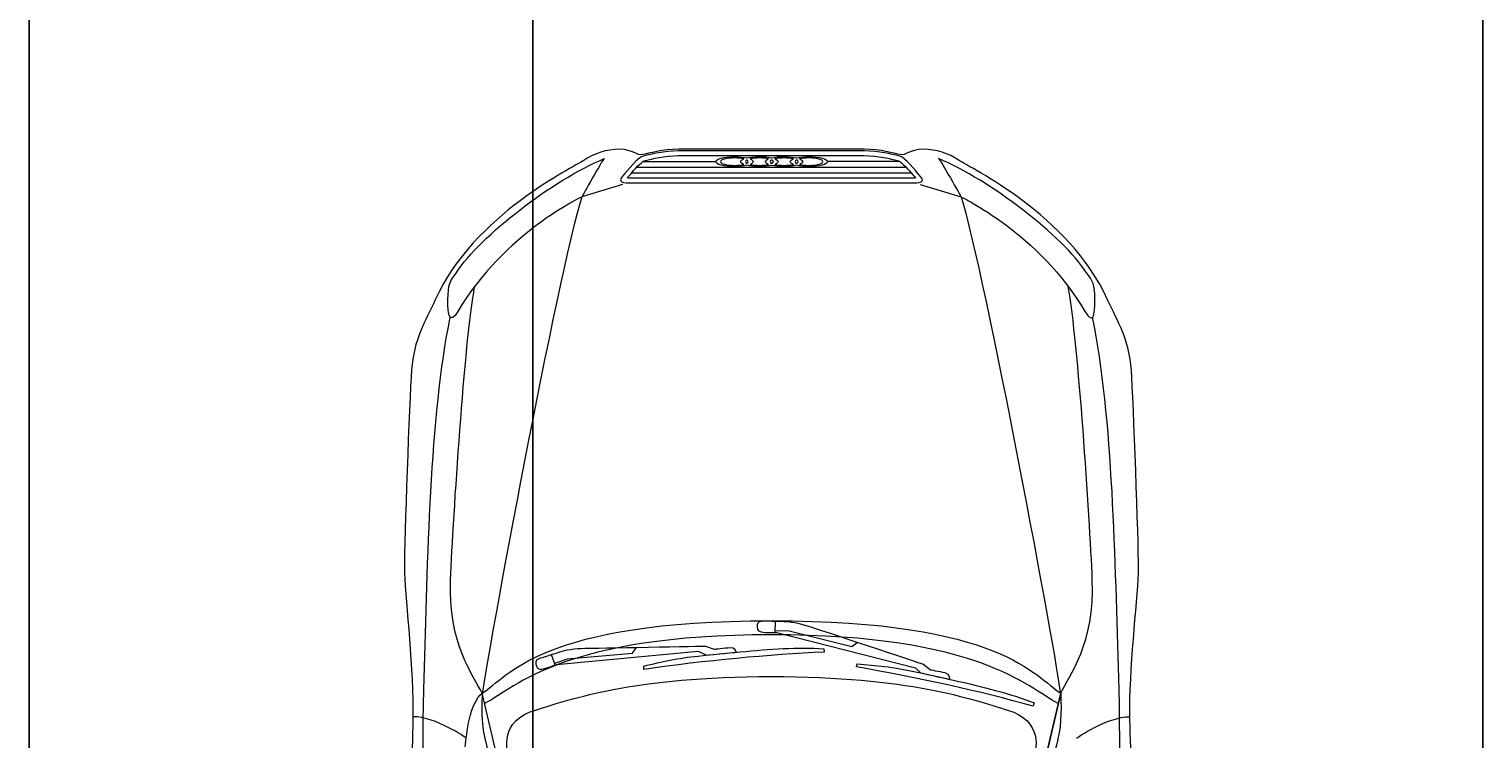
# Model space of a CAD drawing. Units: inches. Extents: x 1734 to 2405, y 1500 to 2491.
# Tile 5 of 14: x 1798 to 1875, y 1851 to 1888. Entities that reach past the tile are written whole.
import ezdxf

# ---------------------------------------------------------------- set-up
doc = ezdxf.new("R2010")
doc.units = ezdxf.units.IN
for name, color, linetype, lineweight in [('A-ANNO-DIMS', 2, 'Continuous', 18), ('AUDI', 8, 'Continuous', 18), ('C-PROP', 7, 'Continuous', 25)]:
    doc.layers.add(name, color=color, linetype=linetype, lineweight=lineweight)
doc.styles.get("Standard").update_dxf_attribs({"font": 'arial.ttf'})
doc.dimstyles.get("Standard").update_dxf_attribs({"dimtxt": 0.18, "dimasz": 0.18, "dimexe": 0.18, "dimexo": 0.0625, "dimgap": 0.09, "dimtad": 0, "dimtih": 1, "dimtoh": 1, "dimdec": 4, "dimzin": 0, "dimdsep": 46, "dimtxsty": 'Standard', "dimcen": 0.09, "dimadec": 0, "dimazin": 0, "dimtfac": 1, "dimtdec": 4, "dimtofl": 0, "dimtmove": 0, "dimatfit": 3, "dimfxl": 1, "dimtolj": 1, "dimtzin": 0, "dimarcsym": 0})

# ---------------------------------------------------------------- blocks, each defined once
blk = doc.blocks.new('*D32')
at = {"layer": 'A-ANNO-DIMS', "color": 0, "lineweight": -2, "transparency": 16777216}
for p, q in [((1798.394, 2202.262), (1798.394, 1615.467)), ((1824.834, 2202.262), (1824.834, 1615.467)), ((1798.574, 1615.647), (1811.219, 1615.647)), ((1824.654, 1615.647), (1812.009, 1615.647))]:
    blk.add_line(p, q, dxfattribs=at)
at = {"layer": 'A-ANNO-DIMS', "color": 0, "transparency": 16777216}
for points in [[(1798.574, 1615.677), (1798.574, 1615.617), (1798.394, 1615.647)], [(1824.654, 1615.677), (1824.654, 1615.617), (1824.834, 1615.647)]]:
    blk.add_solid(points, dxfattribs=at)
at = {"layer": 'Defpoints', "color": 0, "transparency": 16777216}
for p in [(1798.394, 2202.325), (1824.834, 2202.325), (1824.834, 1615.647)]:
    blk.add_point(p, dxfattribs=at)
at = {"layer": 'A-ANNO-DIMS', "color": 0, "transparency": 16777216, "insert": (1811.614, 1615.647), "char_height": 0.18, "attachment_point": 5}
blk.add_mtext('\\A1;26.44', dxfattribs=at)
blk = doc.blocks.new('*D33')
at = {"layer": 'A-ANNO-DIMS', "color": 0, "lineweight": -2, "transparency": 16777216}
for p, q in [((1824.834, 2202.262), (1824.834, 1615.467)), ((1874.676, 2202.262), (1874.676, 1615.467)), ((1825.014, 1615.647), (1849.358, 1615.647)), ((1874.496, 1615.647), (1850.152, 1615.647))]:
    blk.add_line(p, q, dxfattribs=at)
at = {"layer": 'A-ANNO-DIMS', "color": 0, "transparency": 16777216}
for points in [[(1825.014, 1615.677), (1825.014, 1615.617), (1824.834, 1615.647)], [(1874.496, 1615.677), (1874.496, 1615.617), (1874.676, 1615.647)]]:
    blk.add_solid(points, dxfattribs=at)
at = {"layer": 'Defpoints', "color": 0, "transparency": 16777216}
for p in [(1824.834, 2202.325), (1874.676, 2202.325), (1874.676, 1615.647)]:
    blk.add_point(p, dxfattribs=at)
at = {"layer": 'A-ANNO-DIMS', "color": 0, "transparency": 16777216, "insert": (1849.755, 1615.647), "char_height": 0.18, "attachment_point": 5}
blk.add_mtext('\\A1;49.84', dxfattribs=at)

msp = doc.modelspace()

# ---------------------------------------------------------------- linework, layer by layer
at = {"layer": 'AUDI'}
for points, knots in [([(1837.345, 1785.4381), (1823.2241, 1785.5924), (1821.1737, 1790.3408), (1820.3073, 1793.4695), (1820.3073, 1793.4695), (1819.7422, 1795.3167), (1819.2902, 1796.7867), (1819.0641, 1797.5407), (1819.0641, 1797.5407), (1818.838, 1798.2946), (1818.3485, 1800.5941), (1818.3107, 1802.5166), (1818.3107, 1802.5166), (1818.2728, 1804.4391), (1818.0863, 1815.9017), (1818.0863, 1819.0652), (1818.0863, 1819.0652), (1818.0863, 1822.2286), (1818.0863, 1837.0491), (1818.0863, 1839.1573), (1818.0863, 1839.1573), (1818.0863, 1841.2655), (1818.5368, 1849.6746), (1818.5368, 1852.3509), (1818.5368, 1852.3509), (1818.5368, 1855.0274), (1818.0863, 1858.3854), (1818.0863, 1859.7768), (1818.0863, 1859.7768), (1818.0863, 1861.1684), (1818.3482, 1868.5223), (1818.4614, 1870.1433), (1818.4614, 1870.1433), (1818.5745, 1871.7643), (1819.1815, 1872.6836), (1819.7048, 1873.8376), (1819.7048, 1873.8376), (1821.7393, 1878.3231), (1826.9383, 1880.7733), (1827.5035, 1881.1503), (1827.5035, 1881.1503), (1828.0686, 1881.5274), (1828.6686, 1881.7322), (1829.3873, 1881.7322), (1829.3873, 1881.7322), (1830.1059, 1881.7322), (1830.2914, 1881.3766), (1830.5929, 1881.452), (1830.5929, 1881.452), (1830.8943, 1881.5274), (1831.6453, 1881.7322), (1832.4769, 1881.7322), (1832.4769, 1881.7322), (1833.3085, 1881.7322), (1837.345, 1881.7322), (1837.345, 1881.7322), (1837.345, 1881.7322), (1837.345, 1881.7322), (1841.3816, 1881.7322), (1842.2132, 1881.7322), (1842.2132, 1881.7322), (1843.0448, 1881.7322), (1843.7957, 1881.5274), (1844.0972, 1881.452), (1844.0972, 1881.452), (1844.3986, 1881.3766), (1844.5842, 1881.7322), (1845.3028, 1881.7322), (1845.3028, 1881.7322), (1846.0215, 1881.7322), (1846.6215, 1881.5274), (1847.1866, 1881.1503), (1847.1866, 1881.1503), (1847.7517, 1880.7733), (1852.9508, 1878.3231), (1854.9853, 1873.8376), (1854.9853, 1873.8376), (1855.5085, 1872.6836), (1856.1155, 1871.7643), (1856.2287, 1870.1433), (1856.2287, 1870.1433), (1856.3419, 1868.5224), (1856.6038, 1861.1684), (1856.6038, 1859.7768), (1856.6038, 1859.7768), (1856.6038, 1858.3854), (1856.1533, 1855.0274), (1856.1533, 1852.3509), (1856.1533, 1852.3509), (1856.1533, 1849.6746), (1856.6038, 1841.2655), (1856.6038, 1839.1573), (1856.6038, 1839.1573), (1856.6038, 1837.0491), (1856.6038, 1822.2286), (1856.6038, 1819.0652), (1856.6038, 1819.0652), (1856.6038, 1815.9017), (1856.4172, 1804.4391), (1856.3794, 1802.5166), (1856.3794, 1802.5166), (1856.3417, 1800.5941), (1855.8521, 1798.2946), (1855.626, 1797.5407), (1855.626, 1797.5407), (1855.3998, 1796.7867), (1854.9479, 1795.3166), (1854.3827, 1793.4695), (1854.3827, 1793.4695), (1853.5163, 1790.3408), (1851.466, 1785.5924), (1837.345, 1785.4381)], [0, 0, 0, 0, 0.0357143, 0.0357143, 0.0357143, 0.0357143, 0.0714286, 0.0714286, 0.0714286, 0.0714286, 0.1071429, 0.1071429, 0.1071429, 0.1071429, 0.1428571, 0.1428571, 0.1428571, 0.1428572, 0.1785714, 0.1785714, 0.1785714, 0.1785714, 0.2142857, 0.2142857, 0.2142857, 0.2142857, 0.25, 0.25, 0.25, 0.25, 0.2857143, 0.2857143, 0.2857143, 0.2857143, 0.3214286, 0.3214286, 0.3214286, 0.3214286, 0.3571429, 0.3571429, 0.3571429, 0.3571429, 0.3928571, 0.3928571, 0.3928571, 0.3928572, 0.4285714, 0.4285714, 0.4285714, 0.4285714, 0.4642857, 0.4642857, 0.4642857, 0.4642857, 0.5, 0.5, 0.5, 0.5, 0.5357143, 0.5357143, 0.5357143, 0.5357143, 0.5714286, 0.5714286, 0.5714286, 0.5714286, 0.6071429, 0.6071429, 0.6071429, 0.6071429, 0.6428571, 0.6428571, 0.6428571, 0.6428572, 0.6785714, 0.6785714, 0.6785714, 0.6785714, 0.7142857, 0.7142857, 0.7142857, 0.7142857, 0.75, 0.75, 0.75, 0.75, 0.7857143, 0.7857143, 0.7857143, 0.7857143, 0.8214286, 0.8214286, 0.8214286, 0.8214286, 0.8571429, 0.8571429, 0.8571429, 0.8571429, 0.8928571, 0.8928571, 0.8928571, 0.8928572, 0.9285714, 0.9285714, 0.9285714, 0.9285714, 0.9642857, 0.9642857, 0.9642857, 0.9642857, 1, 1, 1, 1]), ([(1820.369, 1873.8468), (1820.369, 1873.0084), (1820.4652, 1872.4997), (1820.895, 1873.2276), (1820.895, 1873.2276), (1823.3094, 1877.3154), (1827.3951, 1879.2352), (1827.3951, 1879.2352), (1827.3951, 1879.2352), (1827.3951, 1879.2353), (1828.502, 1881.2206), (1828.5713, 1881.2483), (1828.5713, 1881.2483), (1825.8757, 1880.1073), (1822.0898, 1877.2323), (1820.8023, 1875.2406), (1820.8023, 1875.2406), (1820.4928, 1874.838), (1820.369, 1874.6372), (1820.369, 1873.8468)], [0, 0, 0, 0, 0.2, 0.2, 0.2, 0.2, 0.4, 0.4, 0.4, 0.4, 0.6, 0.6, 0.6, 0.6, 0.8, 0.8, 0.8, 0.8, 1, 1, 1, 1]), ([(1820.369, 1873.8468), (1820.369, 1873.0084), (1820.4652, 1872.4997), (1820.895, 1873.2276), (1820.895, 1873.2276), (1823.3094, 1877.3154), (1827.3951, 1879.2352), (1827.3951, 1879.2352), (1827.3951, 1879.2352), (1827.3951, 1879.2352), (1828.502, 1881.2206), (1828.5713, 1881.2483), (1828.5713, 1881.2483), (1825.8757, 1880.1073), (1822.0898, 1877.2323), (1820.8023, 1875.2406), (1820.8023, 1875.2406), (1820.4928, 1874.838), (1820.369, 1874.6372), (1820.369, 1873.8468)], [0, 0, 0, 0, 0.2, 0.2, 0.2, 0.2, 0.4, 0.4, 0.4, 0.4, 0.6, 0.6, 0.6, 0.6, 0.8, 0.8, 0.8, 0.8, 1, 1, 1, 1]), ([(1837.4243, 1881.6498), (1837.4243, 1881.6498), (1842.2132, 1881.6498), (1842.2132, 1881.6498), (1842.2132, 1881.6498), (1842.9813, 1881.6498), (1843.6785, 1881.4731), (1844.0134, 1881.3882), (1844.0134, 1881.3882), (1844.0134, 1881.3882), (1844.0772, 1881.3722), (1844.0772, 1881.3722), (1844.0772, 1881.3722), (1844.3817, 1881.2749), (1844.8528, 1880.6621), (1845.1512, 1880.3321), (1845.1512, 1880.3321), (1845.4497, 1880.002), (1845.1512, 1879.9707), (1844.6172, 1879.9707), (1844.6172, 1879.9707), (1844.0832, 1879.9707), (1837.345, 1879.9707), (1837.345, 1879.9707), (1837.345, 1879.9707), (1837.345, 1879.9707), (1830.6069, 1879.9707), (1830.0729, 1879.9707), (1830.0729, 1879.9707), (1829.5389, 1879.9707), (1829.2404, 1880.002), (1829.5389, 1880.3321), (1829.5389, 1880.3321), (1829.8373, 1880.6621), (1830.3084, 1881.2749), (1830.6129, 1881.3722), (1830.6129, 1881.3722), (1830.6129, 1881.3722), (1830.6766, 1881.3883), (1830.6766, 1881.3883), (1830.6766, 1881.3883), (1831.0116, 1881.4731), (1831.7088, 1881.6498), (1832.4769, 1881.6498), (1832.4769, 1881.6498), (1832.4769, 1881.6498), (1837.2658, 1881.6498), (1837.2658, 1881.6498), (1837.2658, 1881.6498), (1837.2658, 1881.6498), (1837.4243, 1881.6498), (1837.4243, 1881.6498)], [0, 0, 0, 0, 0.0769231, 0.0769231, 0.0769231, 0.0769231, 0.1538462, 0.1538462, 0.1538462, 0.1538462, 0.2307692, 0.2307692, 0.2307692, 0.2307692, 0.3076923, 0.3076923, 0.3076923, 0.3076923, 0.3846154, 0.3846154, 0.3846154, 0.3846154, 0.4615385, 0.4615385, 0.4615385, 0.4615385, 0.5384615, 0.5384615, 0.5384615, 0.5384615, 0.6153846, 0.6153846, 0.6153846, 0.6153846, 0.6923077, 0.6923077, 0.6923077, 0.6923077, 0.7692308, 0.7692308, 0.7692308, 0.7692308, 0.8461538, 0.8461538, 0.8461538, 0.8461539, 0.9230769, 0.9230769, 0.9230769, 0.9230769, 1, 1, 1, 1]), ([(1830.0729, 1880.2202), (1830.0729, 1880.2202), (1830.0729, 1880.2202), (1830.0729, 1880.2202), (1830.0729, 1880.2202), (1830.0729, 1880.2202), (1844.6172, 1880.2202), (1844.6172, 1880.2202), (1844.6172, 1880.2202), (1844.74, 1880.2202), (1844.8345, 1880.2232), (1844.9112, 1880.2279), (1844.9112, 1880.2279), (1844.8523, 1880.2953), (1844.7615, 1880.3992), (1844.7615, 1880.3992), (1844.7615, 1880.3992), (1844.5429, 1880.6533), (1844.1773, 1881.0778), (1844.0018, 1881.134), (1844.0018, 1881.134), (1844.0018, 1881.134), (1843.9524, 1881.1463), (1843.9524, 1881.1463), (1843.9524, 1881.1463), (1843.626, 1881.229), (1842.9495, 1881.4005), (1842.2132, 1881.4005), (1842.2132, 1881.4005), (1842.2132, 1881.4005), (1832.4769, 1881.4005), (1832.4769, 1881.4005), (1832.4769, 1881.4005), (1831.7406, 1881.4005), (1831.064, 1881.2289), (1830.7387, 1881.1467), (1830.7387, 1881.1467), (1830.7387, 1881.1467), (1830.6739, 1881.1301), (1830.6739, 1881.1301), (1830.6739, 1881.1301), (1830.5133, 1881.0787), (1830.1474, 1880.6533), (1829.9286, 1880.3992), (1829.9286, 1880.3992), (1829.9286, 1880.3992), (1829.838, 1880.2953), (1829.7789, 1880.2279), (1829.7789, 1880.2279), (1829.8558, 1880.2232), (1829.95, 1880.2202), (1830.0729, 1880.2202)], [0, 0, 0, 0, 0.0769231, 0.0769231, 0.0769231, 0.0769231, 0.1538462, 0.1538462, 0.1538462, 0.1538462, 0.2307692, 0.2307692, 0.2307692, 0.2307692, 0.3076923, 0.3076923, 0.3076923, 0.3076923, 0.3846154, 0.3846154, 0.3846154, 0.3846154, 0.4615385, 0.4615385, 0.4615385, 0.4615385, 0.5384615, 0.5384615, 0.5384615, 0.5384615, 0.6153846, 0.6153846, 0.6153846, 0.6153846, 0.6923077, 0.6923077, 0.6923077, 0.6923077, 0.7692308, 0.7692308, 0.7692308, 0.7692308, 0.8461538, 0.8461538, 0.8461538, 0.8461539, 0.9230769, 0.9230769, 0.9230769, 0.9230769, 1, 1, 1, 1]), ([(1835.4029, 1880.8275), (1835.6563, 1880.8275), (1835.8778, 1880.853), (1836.0518, 1880.8959), (1836.0518, 1880.8959), (1836.2261, 1880.853), (1836.4636, 1880.8274), (1836.717, 1880.8274), (1836.717, 1880.8274), (1836.9701, 1880.8275), (1837.1918, 1880.853), (1837.3659, 1880.8916), (1837.3659, 1880.8916), (1837.5239, 1880.853), (1837.7618, 1880.8274), (1837.9991, 1880.8274), (1837.9991, 1880.8274), (1838.2525, 1880.8275), (1838.49, 1880.853), (1838.6641, 1880.8959), (1838.6641, 1880.8959), (1838.8382, 1880.853), (1839.0598, 1880.8274), (1839.313, 1880.8274), (1839.313, 1880.8274), (1839.8515, 1880.8275), (1840.2947, 1880.9427), (1840.2947, 1881.0876), (1840.2947, 1881.0876), (1840.2947, 1881.2283), (1839.8515, 1881.3481), (1839.313, 1881.3481), (1839.313, 1881.3481), (1839.0598, 1881.3482), (1838.8382, 1881.3182), (1838.6641, 1881.2796), (1838.6641, 1881.2796), (1838.49, 1881.3183), (1838.2525, 1881.3481), (1837.9991, 1881.3481), (1837.9991, 1881.3481), (1837.7618, 1881.3482), (1837.5239, 1881.3225), (1837.3659, 1881.2796), (1837.3659, 1881.2796), (1837.1918, 1881.3226), (1836.9701, 1881.3481), (1836.717, 1881.3481), (1836.717, 1881.3481), (1836.4349, 1881.3482), (1836.1295, 1881.297), (1836.0518, 1881.2796), (1836.0518, 1881.2796), (1835.8778, 1881.3183), (1835.6563, 1881.3481), (1835.4029, 1881.3481), (1835.4029, 1881.3481), (1834.8646, 1881.3482), (1834.4212, 1881.2282), (1834.4212, 1881.0876), (1834.4212, 1881.0876), (1834.4212, 1880.9427), (1834.8646, 1880.8274), (1835.4029, 1880.8275)], [0, 0, 0, 0, 0.0625, 0.0625, 0.0625, 0.0625, 0.125, 0.125, 0.125, 0.125, 0.1875, 0.1875, 0.1875, 0.1875, 0.25, 0.25, 0.25, 0.25, 0.3125, 0.3125, 0.3125, 0.3125, 0.375, 0.375, 0.375, 0.375, 0.4375, 0.4375, 0.4375, 0.4375, 0.5, 0.5, 0.5, 0.5, 0.5625, 0.5625, 0.5625, 0.5625, 0.625, 0.625, 0.625, 0.625, 0.6875, 0.6875, 0.6875, 0.6875, 0.75, 0.75, 0.75, 0.75, 0.8125, 0.8125, 0.8125, 0.8125, 0.875, 0.875, 0.875, 0.875, 0.9375, 0.9375, 0.9375, 0.9375, 1, 1, 1, 1]), ([(1835.4029, 1880.8275), (1835.6563, 1880.8275), (1835.8778, 1880.853), (1836.0518, 1880.8959), (1836.0518, 1880.8959), (1836.2261, 1880.853), (1836.4636, 1880.8274), (1836.717, 1880.8274), (1836.717, 1880.8274), (1836.9701, 1880.8274), (1837.1918, 1880.853), (1837.3659, 1880.8916), (1837.3659, 1880.8916), (1837.5239, 1880.853), (1837.7618, 1880.8274), (1837.9991, 1880.8274), (1837.9991, 1880.8274), (1838.2525, 1880.8274), (1838.49, 1880.853), (1838.6641, 1880.8959), (1838.6641, 1880.8959), (1838.8382, 1880.853), (1839.0598, 1880.8274), (1839.313, 1880.8274), (1839.313, 1880.8274), (1839.8515, 1880.8274), (1840.2947, 1880.9427), (1840.2947, 1881.0876), (1840.2947, 1881.0876), (1840.2947, 1881.2283), (1839.8515, 1881.3481), (1839.313, 1881.3481), (1839.313, 1881.3481), (1839.0598, 1881.3481), (1838.8382, 1881.3182), (1838.6641, 1881.2796), (1838.6641, 1881.2796), (1838.49, 1881.3183), (1838.2525, 1881.3481), (1837.9991, 1881.3481), (1837.9991, 1881.3481), (1837.7618, 1881.3481), (1837.5239, 1881.3225), (1837.3659, 1881.2796), (1837.3659, 1881.2796), (1837.1918, 1881.3226), (1836.9701, 1881.3481), (1836.717, 1881.3481), (1836.717, 1881.3481), (1836.4349, 1881.3481), (1836.1295, 1881.297), (1836.0518, 1881.2796), (1836.0518, 1881.2796), (1835.8778, 1881.3183), (1835.6563, 1881.3481), (1835.4029, 1881.3481), (1835.4029, 1881.3481), (1834.8646, 1881.3481), (1834.4212, 1881.2282), (1834.4212, 1881.0876), (1834.4212, 1881.0876), (1834.4212, 1880.9427), (1834.8646, 1880.8275), (1835.4029, 1880.8275)], [0, 0, 0, 0, 0.0625, 0.0625, 0.0625, 0.0625, 0.125, 0.125, 0.125, 0.125, 0.1875, 0.1875, 0.1875, 0.1875, 0.25, 0.25, 0.25, 0.25, 0.3125, 0.3125, 0.3125, 0.3125, 0.375, 0.375, 0.375, 0.375, 0.4375, 0.4375, 0.4375, 0.4375, 0.5, 0.5, 0.5, 0.5, 0.5625, 0.5625, 0.5625, 0.5625, 0.625, 0.625, 0.625, 0.625, 0.6875, 0.6875, 0.6875, 0.6875, 0.75, 0.75, 0.75, 0.75, 0.8125, 0.8125, 0.8125, 0.8125, 0.875, 0.875, 0.875, 0.875, 0.9375, 0.9375, 0.9375, 0.9375, 1, 1, 1, 1]), ([(1835.4029, 1881.2796), (1835.5927, 1881.2796), (1835.7671, 1881.2626), (1835.8937, 1881.2282), (1835.8937, 1881.2282), (1835.7986, 1881.1858), (1835.7352, 1881.1389), (1835.7352, 1881.0876), (1835.7352, 1881.0876), (1835.7352, 1881.0323), (1835.7986, 1880.9854), (1835.8937, 1880.9427), (1835.8937, 1880.9427), (1835.7671, 1880.9129), (1835.5927, 1880.8916), (1835.4029, 1880.8916), (1835.4029, 1880.8916), (1834.9912, 1880.8916), (1834.6746, 1880.9768), (1834.6746, 1881.0876), (1834.6746, 1881.0876), (1834.6746, 1881.1943), (1834.9912, 1881.2796), (1835.4029, 1881.2796)], [0, 0, 0, 0, 0.1666667, 0.1666667, 0.1666667, 0.1666667, 0.3333333, 0.3333333, 0.3333333, 0.3333333, 0.5, 0.5, 0.5, 0.5, 0.6666667, 0.6666667, 0.6666667, 0.6666667, 0.8333333, 0.8333333, 0.8333333, 0.8333333, 1, 1, 1, 1]), ([(1836.1312, 1881.0877), (1836.1312, 1881.0535), (1836.0995, 1881.0279), (1836.0518, 1881.0024), (1836.0518, 1881.0024), (1836.0046, 1881.028), (1835.9887, 1881.0535), (1835.9887, 1881.0876), (1835.9887, 1881.0876), (1835.9887, 1881.1177), (1836.0046, 1881.1473), (1836.0518, 1881.1731), (1836.0518, 1881.1731), (1836.0995, 1881.1473), (1836.1312, 1881.1177), (1836.1312, 1881.0877)], [0, 0, 0, 0, 0.25, 0.25, 0.25, 0.25, 0.5, 0.5, 0.5, 0.5, 0.75, 0.75, 0.75, 0.75, 1, 1, 1, 1]), ([(1837.1918, 1881.2326), (1837.0966, 1881.1901), (1837.0335, 1881.1389), (1837.0335, 1881.0876), (1837.0335, 1881.0876), (1837.0335, 1881.0323), (1837.0966, 1880.9811), (1837.1918, 1880.9384), (1837.1918, 1880.9384), (1837.0653, 1880.9086), (1836.9068, 1880.8916), (1836.717, 1880.8916), (1836.717, 1880.8916), (1836.5267, 1880.8916), (1836.3528, 1880.9129), (1836.2261, 1880.9427), (1836.2261, 1880.9427), (1836.321, 1880.9855), (1836.3844, 1881.0322), (1836.3844, 1881.0876), (1836.3844, 1881.0876), (1836.3844, 1881.139), (1836.321, 1881.1858), (1836.2261, 1881.2282), (1836.2261, 1881.2282), (1836.3528, 1881.2627), (1836.5267, 1881.2796), (1836.717, 1881.2796), (1836.717, 1881.2796), (1836.9068, 1881.2796), (1837.0653, 1881.2626), (1837.1918, 1881.2326)], [0, 0, 0, 0, 0.125, 0.125, 0.125, 0.125, 0.25, 0.25, 0.25, 0.25, 0.375, 0.375, 0.375, 0.375, 0.5, 0.5, 0.5, 0.5, 0.625, 0.625, 0.625, 0.625, 0.75, 0.75, 0.75, 0.75, 0.875, 0.875, 0.875, 0.875, 1, 1, 1, 1]), ([(1837.4449, 1881.0877), (1837.4449, 1881.0535), (1837.4135, 1881.0236), (1837.3659, 1880.9938), (1837.3659, 1880.9938), (1837.3025, 1881.0237), (1837.271, 1881.0535), (1837.271, 1881.0876), (1837.271, 1881.0876), (1837.271, 1881.1177), (1837.3025, 1881.1516), (1837.3659, 1881.1774), (1837.3659, 1881.1774), (1837.4135, 1881.1517), (1837.4449, 1881.1177), (1837.4449, 1881.0877)], [0, 0, 0, 0, 0.25, 0.25, 0.25, 0.25, 0.5, 0.5, 0.5, 0.5, 0.75, 0.75, 0.75, 0.75, 1, 1, 1, 1]), ([(1838.5056, 1881.2283), (1838.3948, 1881.1858), (1838.3317, 1881.1389), (1838.3317, 1881.0876), (1838.3317, 1881.0876), (1838.3317, 1881.0323), (1838.3948, 1880.9854), (1838.5056, 1880.9427), (1838.5056, 1880.9427), (1838.3632, 1880.9129), (1838.1891, 1880.8916), (1837.9991, 1880.8916), (1837.9991, 1880.8916), (1837.8249, 1880.8916), (1837.6508, 1880.9086), (1837.5239, 1880.9384), (1837.5239, 1880.9384), (1837.6351, 1880.9812), (1837.6983, 1881.0322), (1837.6983, 1881.0876), (1837.6983, 1881.0876), (1837.6983, 1881.139), (1837.6351, 1881.19), (1837.5239, 1881.2325), (1837.5239, 1881.2325), (1837.6508, 1881.2627), (1837.8249, 1881.2796), (1837.9991, 1881.2796), (1837.9991, 1881.2796), (1838.1891, 1881.2796), (1838.3632, 1881.2626), (1838.5056, 1881.2283)], [0, 0, 0, 0, 0.125, 0.125, 0.125, 0.125, 0.25, 0.25, 0.25, 0.25, 0.375, 0.375, 0.375, 0.375, 0.5, 0.5, 0.5, 0.5, 0.625, 0.625, 0.625, 0.625, 0.75, 0.75, 0.75, 0.75, 0.875, 0.875, 0.875, 0.875, 1, 1, 1, 1]), ([(1838.7431, 1881.0877), (1838.7431, 1881.0535), (1838.7115, 1881.0279), (1838.6641, 1881.0024), (1838.6641, 1881.0024), (1838.6164, 1881.028), (1838.5848, 1881.0535), (1838.5848, 1881.0876), (1838.5848, 1881.0876), (1838.5848, 1881.1177), (1838.6164, 1881.1473), (1838.6641, 1881.1731), (1838.6641, 1881.1731), (1838.7115, 1881.1473), (1838.7431, 1881.1177), (1838.7431, 1881.0877)], [0, 0, 0, 0, 0.25, 0.25, 0.25, 0.25, 0.5, 0.5, 0.5, 0.5, 0.75, 0.75, 0.75, 0.75, 1, 1, 1, 1]), ([(1840.0413, 1881.0877), (1840.0413, 1880.9769), (1839.7248, 1880.8916), (1839.313, 1880.8916), (1839.313, 1880.8916), (1839.1231, 1880.8916), (1838.949, 1880.9129), (1838.8223, 1880.9427), (1838.8223, 1880.9427), (1838.9175, 1880.9855), (1838.9806, 1881.0322), (1838.9806, 1881.0876), (1838.9806, 1881.0876), (1838.9806, 1881.139), (1838.9175, 1881.1858), (1838.8223, 1881.2282), (1838.8223, 1881.2282), (1838.949, 1881.2627), (1839.1231, 1881.2796), (1839.313, 1881.2796), (1839.313, 1881.2796), (1839.7248, 1881.2796), (1840.0413, 1881.1943), (1840.0413, 1881.0877)], [0, 0, 0, 0, 0.1666667, 0.1666667, 0.1666667, 0.1666667, 0.3333333, 0.3333333, 0.3333333, 0.3333333, 0.5, 0.5, 0.5, 0.5, 0.6666667, 0.6666667, 0.6666667, 0.6666667, 0.8333333, 0.8333333, 0.8333333, 0.8333333, 1, 1, 1, 1]), ([(1854.3211, 1873.8468), (1854.3211, 1873.0084), (1854.2249, 1872.4997), (1853.7951, 1873.2276), (1853.7951, 1873.2276), (1851.3807, 1877.3154), (1847.295, 1879.2352), (1847.295, 1879.2352), (1847.295, 1879.2352), (1847.295, 1879.2353), (1846.1881, 1881.2206), (1846.1187, 1881.2483), (1846.1187, 1881.2483), (1848.8144, 1880.1073), (1852.6003, 1877.2323), (1853.8878, 1875.2406), (1853.8878, 1875.2406), (1854.1972, 1874.838), (1854.3211, 1874.6372), (1854.3211, 1873.8468)], [0, 0, 0, 0, 0.2, 0.2, 0.2, 0.2, 0.4, 0.4, 0.4, 0.4, 0.6, 0.6, 0.6, 0.6, 0.8, 0.8, 0.8, 0.8, 1, 1, 1, 1]), ([(1854.3211, 1873.8468), (1854.3211, 1873.0084), (1854.2249, 1872.4997), (1853.7951, 1873.2276), (1853.7951, 1873.2276), (1851.3807, 1877.3154), (1847.295, 1879.2352), (1847.295, 1879.2352), (1847.295, 1879.2352), (1847.295, 1879.2352), (1846.1881, 1881.2206), (1846.1187, 1881.2483), (1846.1187, 1881.2483), (1848.8144, 1880.1073), (1852.6003, 1877.2323), (1853.8878, 1875.2406), (1853.8878, 1875.2406), (1854.1972, 1874.838), (1854.3211, 1874.6372), (1854.3211, 1873.8468)], [0, 0, 0, 0, 0.2, 0.2, 0.2, 0.2, 0.4, 0.4, 0.4, 0.4, 0.6, 0.6, 0.6, 0.6, 0.8, 0.8, 0.8, 0.8, 1, 1, 1, 1]), ([(1822.1668, 1853.1904), (1821.7271, 1854.0704), (1820.3628, 1855.8263), (1820.5081, 1859.1446), (1820.5081, 1859.1446), (1820.6535, 1862.463), (1821.2427, 1871.6184), (1821.7713, 1874.5311)], [0, 0, 0, 0, 0.5, 0.5, 0.5, 0.5, 1, 1, 1, 1]), ([(1852.5232, 1853.1904), (1852.963, 1854.0704), (1854.3273, 1855.8263), (1854.182, 1859.1446), (1854.182, 1859.1446), (1854.0366, 1862.463), (1853.4474, 1871.6184), (1852.9188, 1874.5311)], [0, 0, 0, 0, 0.5, 0.5, 0.5, 0.5, 1, 1, 1, 1]), ([(1820.9696, 1793.4282), (1820.2601, 1796.9777), (1819.5047, 1804.1661), (1819.3757, 1811.6524), (1819.3757, 1811.6524), (1819.2466, 1819.1387), (1818.9243, 1847.9218), (1819.1178, 1853.9881), (1819.1178, 1853.9881), (1819.3112, 1860.0545), (1819.4195, 1867.7073), (1820.4941, 1872.916)], [0, 0, 0, 0, 0.3333333, 0.3333333, 0.3333333, 0.3333333, 0.6666667, 0.6666667, 0.6666667, 0.6666667, 1, 1, 1, 1]), ([(1853.7205, 1793.4282), (1854.43, 1796.9777), (1855.1854, 1804.1661), (1855.3144, 1811.6524), (1855.3144, 1811.6524), (1855.4435, 1819.1387), (1855.7658, 1847.9218), (1855.5723, 1853.9881), (1855.5723, 1853.9881), (1855.3788, 1860.0545), (1855.2706, 1867.7073), (1854.1959, 1872.916)], [0, 0, 0, 0, 0.3333333, 0.3333333, 0.3333333, 0.3333333, 0.6666667, 0.6666667, 0.6666667, 0.6666667, 1, 1, 1, 1]), ([(1837.345, 1839.9913), (1843.7369, 1839.9913), (1849.1528, 1838.8351), (1849.1528, 1838.8351), (1849.1528, 1838.8351), (1849.1528, 1838.8351), (1852.5232, 1853.1904), (1852.5232, 1853.1904), (1852.5232, 1853.1904), (1851.175, 1854.0577), (1849.4184, 1856.9963), (1837.345, 1856.9963), (1837.345, 1856.9963), (1825.2717, 1856.9963), (1823.515, 1854.0577), (1822.1669, 1853.1904), (1822.1669, 1853.1904), (1822.1669, 1853.1904), (1825.5373, 1838.8351), (1825.5373, 1838.8351), (1825.5373, 1838.8351), (1825.5373, 1838.8351), (1830.9532, 1839.9913), (1837.345, 1839.9913)], [0, 0, 0, 0, 0.1666667, 0.1666667, 0.1666667, 0.1666667, 0.3333333, 0.3333333, 0.3333333, 0.3333333, 0.5, 0.5, 0.5, 0.5, 0.6666667, 0.6666667, 0.6666667, 0.6666667, 0.8333333, 0.8333333, 0.8333333, 0.8333333, 1, 1, 1, 1]), ([(1837.345, 1839.9913), (1843.7369, 1839.9913), (1849.1528, 1838.8351), (1849.1528, 1838.8351), (1849.1528, 1838.8351), (1849.1528, 1838.8351), (1852.5232, 1853.1904), (1852.5232, 1853.1904), (1852.5232, 1853.1904), (1851.175, 1854.0577), (1849.4184, 1856.9963), (1837.345, 1856.9963), (1837.345, 1856.9963), (1825.2717, 1856.9963), (1823.515, 1854.0577), (1822.1669, 1853.1904), (1822.1669, 1853.1904), (1822.1669, 1853.1904), (1825.5373, 1838.8351), (1825.5373, 1838.8351), (1825.5373, 1838.8351), (1825.5373, 1838.8351), (1830.9532, 1839.9913), (1837.345, 1839.9913)], [0, 0, 0, 0, 0.1666667, 0.1666667, 0.1666667, 0.1666667, 0.3333333, 0.3333333, 0.3333333, 0.3333333, 0.5, 0.5, 0.5, 0.5, 0.6666667, 0.6666667, 0.6666667, 0.6666667, 0.8333333, 0.8333333, 0.8333333, 0.8333333, 1, 1, 1, 1]), ([(1837.7824, 1856.9464), (1838.3682, 1856.9464), (1838.7955, 1856.8512), (1839.3023, 1856.6928), (1839.3023, 1856.6928), (1839.6821, 1856.582), (1845.286, 1854.7128), (1845.286, 1854.7128), (1845.286, 1854.7128), (1845.286, 1854.7128), (1845.6661, 1854.4118), (1845.6661, 1854.4118), (1845.6661, 1854.4118), (1845.6661, 1854.4118), (1846.1726, 1854.3169), (1846.4576, 1854.2537), (1846.4576, 1854.2537), (1846.7427, 1854.1746), (1846.711, 1853.9209), (1846.711, 1853.9209), (1846.711, 1853.9209), (1846.711, 1853.9209), (1845.1594, 1854.2694), (1845.1594, 1854.2694), (1845.1594, 1854.2694), (1845.1594, 1854.2694), (1844.9062, 1854.523), (1844.9062, 1854.523), (1844.9062, 1854.523), (1844.9062, 1854.523), (1837.624, 1856.3761), (1837.624, 1856.3761), (1837.624, 1856.3761), (1837.624, 1856.3761), (1837.3865, 1856.376), (1837.0223, 1856.376), (1837.0223, 1856.376), (1836.6581, 1856.3918), (1836.595, 1856.5186), (1836.595, 1856.661), (1836.595, 1856.661), (1836.595, 1856.8195), (1836.6109, 1856.9623), (1836.8325, 1856.9623), (1836.8325, 1856.9623), (1837.0541, 1856.978), (1837.4182, 1856.9623), (1837.7824, 1856.9464)], [0, 0, 0, 0, 0.0833333, 0.0833333, 0.0833333, 0.0833333, 0.1666667, 0.1666667, 0.1666667, 0.1666667, 0.25, 0.25, 0.25, 0.25, 0.3333333, 0.3333333, 0.3333333, 0.3333333, 0.4166667, 0.4166667, 0.4166667, 0.4166667, 0.5, 0.5, 0.5, 0.5, 0.5833333, 0.5833333, 0.5833333, 0.5833333, 0.6666667, 0.6666667, 0.6666667, 0.6666667, 0.75, 0.75, 0.75, 0.75, 0.8333333, 0.8333333, 0.8333333, 0.8333333, 0.9166667, 0.9166667, 0.9166667, 0.9166667, 1, 1, 1, 1]), ([(1852.3959, 1852.6485), (1850.7544, 1853.5213), (1848.2176, 1856.2553), (1837.345, 1856.2553), (1837.345, 1856.2553), (1826.4724, 1856.2553), (1823.9357, 1853.5213), (1822.2942, 1852.6484)], [0, 0, 0, 0, 0.5, 0.5, 0.5, 0.5, 1, 1, 1, 1]), ([(1837.545, 1856.4869), (1837.545, 1856.4869), (1838.2731, 1856.471), (1838.2731, 1856.471), (1838.2731, 1856.471), (1838.2731, 1856.471), (1841.5658, 1855.6473), (1841.5658, 1855.6473), (1841.5658, 1855.6473), (1841.5658, 1855.6473), (1841.8351, 1855.8532), (1841.8351, 1855.8532)], [0, 0, 0, 0, 0.3333333, 0.3333333, 0.3333333, 0.3333333, 0.6666667, 0.6666667, 0.6666667, 0.6666667, 1, 1, 1, 1]), ([(1826.0357, 1855.2829), (1826.574, 1855.4732), (1827.0172, 1855.5206), (1827.5555, 1855.5365), (1827.5555, 1855.5365), (1827.9512, 1855.5365), (1833.9037, 1855.6473), (1833.9037, 1855.6473), (1833.9037, 1855.6473), (1833.9037, 1855.6473), (1834.3627, 1855.4888), (1834.3627, 1855.4888), (1834.3627, 1855.4888), (1834.3627, 1855.4888), (1834.8852, 1855.5524), (1835.1701, 1855.5683), (1835.1701, 1855.5683), (1835.4553, 1855.5999), (1835.5025, 1855.3464), (1835.5025, 1855.3464), (1835.5025, 1855.3464), (1835.5025, 1855.3464), (1833.9355, 1855.188), (1833.9355, 1855.188), (1833.9355, 1855.188), (1833.9355, 1855.188), (1833.508, 1855.3939), (1833.508, 1855.3939), (1833.508, 1855.3939), (1833.508, 1855.3939), (1826.0674, 1854.6969), (1826.0674, 1854.6969), (1826.0674, 1854.6969), (1826.0674, 1854.6969), (1825.8459, 1854.6179), (1825.4976, 1854.5071), (1825.4976, 1854.5071), (1825.165, 1854.3961), (1825.0542, 1854.4912), (1825.0067, 1854.6338), (1825.0067, 1854.6338), (1824.959, 1854.7919), (1824.9275, 1854.9192), (1825.1334, 1854.998), (1825.1334, 1854.998), (1825.3391, 1855.0614), (1825.6874, 1855.1721), (1826.0357, 1855.2829)], [0, 0, 0, 0, 0.0833333, 0.0833333, 0.0833333, 0.0833333, 0.1666667, 0.1666667, 0.1666667, 0.1666667, 0.25, 0.25, 0.25, 0.25, 0.3333333, 0.3333333, 0.3333333, 0.3333333, 0.4166667, 0.4166667, 0.4166667, 0.4166667, 0.5, 0.5, 0.5, 0.5, 0.5833333, 0.5833333, 0.5833333, 0.5833333, 0.6666667, 0.6666667, 0.6666667, 0.6666667, 0.75, 0.75, 0.75, 0.75, 0.8333333, 0.8333333, 0.8333333, 0.8333333, 0.9166667, 0.9166667, 0.9166667, 0.9166667, 1, 1, 1, 1]), ([(1826.0357, 1855.2829), (1826.574, 1855.4732), (1827.0172, 1855.5206), (1827.5555, 1855.5365), (1827.5555, 1855.5365), (1827.9512, 1855.5365), (1833.9037, 1855.6473), (1833.9037, 1855.6473), (1833.9037, 1855.6473), (1833.9037, 1855.6473), (1834.3627, 1855.4888), (1834.3627, 1855.4888), (1834.3627, 1855.4888), (1834.3627, 1855.4888), (1834.8852, 1855.5524), (1835.1701, 1855.5683), (1835.1701, 1855.5683), (1835.4553, 1855.5999), (1835.5025, 1855.3464), (1835.5025, 1855.3464), (1835.5025, 1855.3464), (1835.5025, 1855.3464), (1833.9355, 1855.188), (1833.9355, 1855.188), (1833.9355, 1855.188), (1833.9355, 1855.188), (1833.508, 1855.3939), (1833.508, 1855.3939), (1833.508, 1855.3939), (1833.508, 1855.3939), (1826.0674, 1854.6969), (1826.0674, 1854.6969), (1826.0674, 1854.6969), (1826.0674, 1854.6969), (1825.8459, 1854.6179), (1825.4976, 1854.5071), (1825.4976, 1854.5071), (1825.165, 1854.3961), (1825.0542, 1854.4912), (1825.0067, 1854.6338), (1825.0067, 1854.6338), (1824.959, 1854.7919), (1824.9275, 1854.9192), (1825.1334, 1854.998), (1825.1334, 1854.998), (1825.3391, 1855.0614), (1825.6874, 1855.1721), (1826.0357, 1855.2829)], [0, 0, 0, 0, 0.0833333, 0.0833333, 0.0833333, 0.0833333, 0.1666667, 0.1666667, 0.1666667, 0.1666667, 0.25, 0.25, 0.25, 0.25, 0.3333333, 0.3333333, 0.3333333, 0.3333333, 0.4166667, 0.4166667, 0.4166667, 0.4166667, 0.5, 0.5, 0.5, 0.5, 0.5833333, 0.5833333, 0.5833333, 0.5833333, 0.6666667, 0.6666667, 0.6666667, 0.6666667, 0.75, 0.75, 0.75, 0.75, 0.8333333, 0.8333333, 0.8333333, 0.8333333, 0.9166667, 0.9166667, 0.9166667, 0.9166667, 1, 1, 1, 1]), ([(1825.9725, 1854.7762), (1825.9725, 1854.7762), (1826.653, 1854.998), (1826.653, 1854.998), (1826.653, 1854.998), (1826.653, 1854.998), (1830.0568, 1855.2988), (1830.0568, 1855.2988), (1830.0568, 1855.2988), (1830.0568, 1855.2988), (1830.2468, 1855.5683), (1830.2468, 1855.5683)], [0, 0, 0, 0, 0.3333333, 0.3333333, 0.3333333, 0.3333333, 0.6666667, 0.6666667, 0.6666667, 0.6666667, 1, 1, 1, 1]), ([(1840.0937, 1855.5206), (1838.7322, 1855.6156), (1837.2439, 1855.5047), (1835.7083, 1855.3623), (1835.7083, 1855.3623), (1834.9644, 1855.2829), (1834.2202, 1855.2198), (1833.4921, 1855.1403), (1833.4921, 1855.1403), (1832.4632, 1855.0455), (1831.5925, 1854.8395), (1830.6425, 1854.6179), (1830.6425, 1854.6179), (1830.6425, 1854.6179), (1830.6425, 1854.4434), (1830.6425, 1854.4434), (1830.6425, 1854.4434), (1833.8719, 1854.9031), (1837.2282, 1855.2198), (1840.1096, 1855.3464), (1840.1096, 1855.3464), (1840.1096, 1855.3464), (1840.0937, 1855.5206), (1840.0937, 1855.5206)], [0, 0, 0, 0, 0.1666667, 0.1666667, 0.1666667, 0.1666667, 0.3333333, 0.3333333, 0.3333333, 0.3333333, 0.5, 0.5, 0.5, 0.5, 0.6666667, 0.6666667, 0.6666667, 0.6666667, 0.8333333, 0.8333333, 0.8333333, 0.8333333, 1, 1, 1, 1]), ([(1851.1278, 1852.6855), (1849.8613, 1853.1763), (1848.4206, 1853.5406), (1846.9008, 1853.8732), (1846.9008, 1853.8732), (1846.1726, 1854.0317), (1845.4445, 1854.2059), (1844.7321, 1854.3484), (1844.7321, 1854.3484), (1843.7347, 1854.5707), (1842.8322, 1854.6494), (1841.851, 1854.7287), (1841.851, 1854.7287), (1841.851, 1854.7287), (1841.8033, 1854.5707), (1841.8033, 1854.5707), (1841.8033, 1854.5707), (1845.017, 1854.0159), (1848.2941, 1853.2873), (1851.0803, 1852.5113), (1851.0803, 1852.5113), (1851.0803, 1852.5113), (1851.1278, 1852.6855), (1851.1278, 1852.6855)], [0, 0, 0, 0, 0.1666667, 0.1666667, 0.1666667, 0.1666667, 0.3333333, 0.3333333, 0.3333333, 0.3333333, 0.5, 0.5, 0.5, 0.5, 0.6666667, 0.6666667, 0.6666667, 0.6666667, 0.8333333, 0.8333333, 0.8333333, 0.8333333, 1, 1, 1, 1]), ([(1837.345, 1840.8946), (1842.4186, 1840.8946), (1846.5714, 1840.0626), (1847.5327, 1839.9172), (1847.5327, 1839.9172), (1848.3171, 1839.7985), (1849.0424, 1840.6471), (1849.2623, 1841.6646), (1849.2623, 1841.6646), (1849.4821, 1842.682), (1850.8838, 1848.6218), (1851.0763, 1849.4743), (1851.0763, 1849.4743), (1851.2687, 1850.3268), (1851.5984, 1851.7292), (1849.7295, 1852.3066), (1849.7295, 1852.3066), (1847.8606, 1852.8843), (1844.5569, 1854.0665), (1837.345, 1854.0665), (1837.345, 1854.0665), (1830.1332, 1854.0665), (1826.8295, 1852.8842), (1824.9606, 1852.3066), (1824.9606, 1852.3066), (1823.0916, 1851.7293), (1823.4214, 1850.3267), (1823.6138, 1849.4743), (1823.6138, 1849.4743), (1823.8062, 1848.6218), (1825.2079, 1842.682), (1825.4278, 1841.6646), (1825.4278, 1841.6646), (1825.6477, 1840.6471), (1826.373, 1839.7985), (1827.1574, 1839.9172), (1827.1574, 1839.9172), (1828.1187, 1840.0626), (1832.2714, 1840.8946), (1837.345, 1840.8946)], [0, 0, 0, 0, 0.1, 0.1, 0.1, 0.1, 0.2, 0.2, 0.2, 0.2, 0.3, 0.3, 0.3, 0.3, 0.4, 0.4, 0.4, 0.4, 0.5, 0.5, 0.5, 0.5, 0.6, 0.6, 0.6, 0.6, 0.7, 0.7, 0.7, 0.7, 0.8, 0.8, 0.8, 0.8, 0.9, 0.9, 0.9, 0.9, 1, 1, 1, 1]), ([(1822.1668, 1853.1904), (1822.1668, 1853.1904), (1825.5373, 1838.8351), (1825.5373, 1838.8351), (1825.5373, 1838.8351), (1825.5373, 1838.8351), (1825.0104, 1839.3572), (1824.8178, 1840.1762), (1824.8178, 1840.1762), (1824.6251, 1840.9952), (1822.3895, 1850.352), (1822.245, 1851.1227), (1822.245, 1851.1227), (1822.1005, 1851.8934), (1822.1669, 1853.1904), (1822.1668, 1853.1904)], [0, 0, 0, 0, 0.25, 0.25, 0.25, 0.25, 0.5, 0.5, 0.5, 0.5, 0.75, 0.75, 0.75, 0.75, 1, 1, 1, 1]), ([(1822.1668, 1853.1904), (1822.1668, 1853.1904), (1825.5373, 1838.8351), (1825.5373, 1838.8351), (1825.5373, 1838.8351), (1825.5373, 1838.8351), (1825.0104, 1839.3572), (1824.8178, 1840.1762), (1824.8178, 1840.1762), (1824.6251, 1840.9952), (1822.3895, 1850.352), (1822.245, 1851.1227), (1822.245, 1851.1227), (1822.1005, 1851.8934), (1822.1668, 1853.1904), (1822.1668, 1853.1904)], [0, 0, 0, 0, 0.25, 0.25, 0.25, 0.25, 0.5, 0.5, 0.5, 0.5, 0.75, 0.75, 0.75, 0.75, 1, 1, 1, 1]), ([(1852.5232, 1853.1904), (1852.5232, 1853.1904), (1849.1528, 1838.8351), (1849.1528, 1838.8351), (1849.1528, 1838.8351), (1849.1528, 1838.8351), (1849.6797, 1839.3572), (1849.8723, 1840.1762), (1849.8723, 1840.1762), (1850.0649, 1840.9952), (1852.3006, 1850.352), (1852.4451, 1851.1227), (1852.4451, 1851.1227), (1852.5896, 1851.8934), (1852.5232, 1853.1904), (1852.5232, 1853.1904)], [0, 0, 0, 0, 0.25, 0.25, 0.25, 0.25, 0.5, 0.5, 0.5, 0.5, 0.75, 0.75, 0.75, 0.75, 1, 1, 1, 1])]:
    msp.add_open_spline(points, degree=3, knots=knots, dxfattribs=at)
for points in [[(1830.0093, 1880.4929), (1830.0093, 1880.4929), (1844.6636, 1880.4929), (1844.6636, 1880.4929)], [(1830.2871, 1880.8023), (1830.2871, 1880.8023), (1844.3621, 1880.8023), (1844.3621, 1880.8023)], [(1830.6127, 1881.0986), (1830.6127, 1881.0986), (1834.4212, 1881.0986), (1834.4212, 1881.0986)], [(1844.0774, 1881.0986), (1844.0774, 1881.0986), (1840.2689, 1881.0986), (1840.2689, 1881.0986)], [(1829.5339, 1879.8925), (1829.5339, 1879.8925), (1827.3951, 1879.2353), (1827.3951, 1879.2353)], [(1845.1562, 1879.8925), (1845.1562, 1879.8925), (1847.295, 1879.2353), (1847.295, 1879.2353)], [(1827.3951, 1879.2353), (1826.1517, 1875.2775), (1822.3801, 1855.0016), (1822.1602, 1853.0217)], [(1847.295, 1879.2353), (1848.5384, 1875.2775), (1852.31, 1855.0016), (1852.5299, 1853.0217)], [(1837.545, 1856.3761), (1837.545, 1856.3761), (1837.5606, 1856.9623), (1837.5606, 1856.9623)], [(1826.0041, 1854.6654), (1826.0041, 1854.6654), (1825.8138, 1855.2198), (1825.8138, 1855.2198)], [(1821.2776, 1850.3817), (1821.3509, 1851.0418), (1821.5068, 1852.6837), (1822.1669, 1853.1904)], [(1821.3303, 1850.8427), (1821.3303, 1850.8427), (1819.7485, 1851.9579), (1818.5342, 1851.9579)], [(1853.3598, 1850.8427), (1853.3598, 1850.8427), (1854.9417, 1851.9579), (1856.1559, 1851.9579)]]:
    msp.add_open_spline(points, degree=3, dxfattribs=at)
at = {"layer": 'C-PROP'}
msp.add_line((1798.3942, 1900.8246), (1798.3942, 1710.7667), dxfattribs=at)

# ---------------------------------------------------------------- dimensions: what is measured, and where the dimension line sits
at = {"layer": 'A-ANNO-DIMS'}
for base, p1, p2, picture, middle in [((1824.8343, 1615.6468), (1798.3942, 2202.3246), (1824.8343, 2202.3246), '*D32', (1811.6142, 1615.6468)), ((1874.676, 1615.6468), (1824.8343, 2202.3246), (1874.676, 2202.3246), '*D33', (1849.7551, 1615.6468))]:
    dim = msp.add_linear_dim(base=base, p1=p1, p2=p2, dimstyle='Standard', override={"dimdec": 2, "dimlfac": 1, "dimrnd": 0, "dimzin": 0, "dimdsep": 46, "dimlunit": 2}, dxfattribs=at)
    dim.commit()
    dim.dimension.update_dxf_attribs({"geometry": picture, "text_midpoint": middle})

doc.saveas('drawing.dxf')
